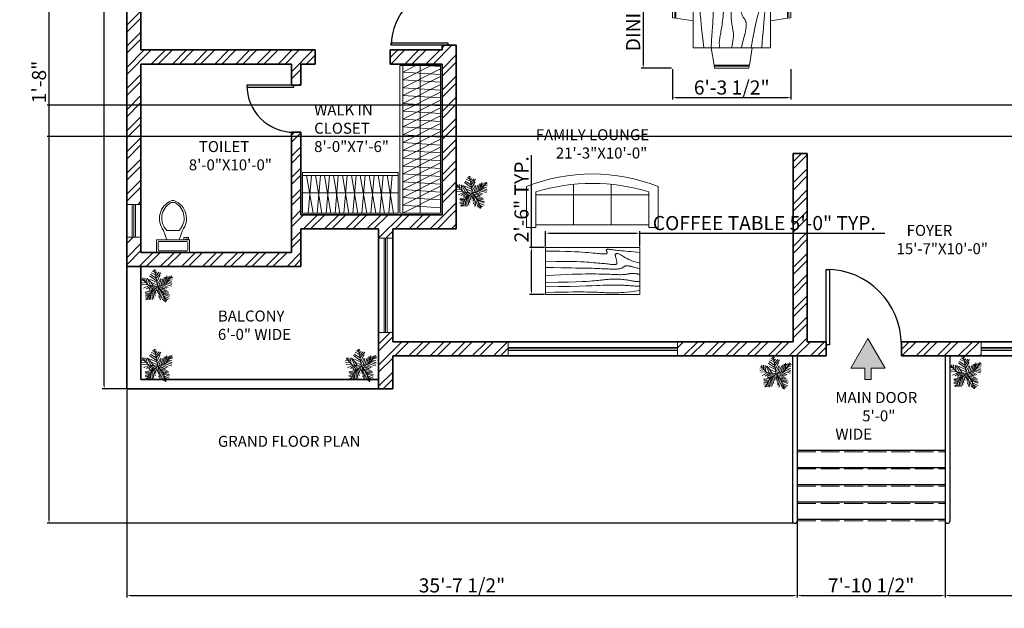
# Model space of a CAD drawing. Units: inches. Extents: x 416 to 1422, y 799 to 1634.
# Tile 1 of 5: x 416 to 1043, y 799 to 1174. Entities that reach past the tile are written whole.
import ezdxf

# ---------------------------------------------------------------- set-up
doc = ezdxf.new("R2010")
doc.units = ezdxf.units.IN
doc.linetypes.add('ACAD_ISO02W100', pattern=[15, 12, -3])
for name, color, linetype, lineweight in [('A-ANNO-DIMS', 2, 'Continuous', 18), ('A-ANNO-SYMB', 7, 'Continuous', 18), ('A-ANNO-TEXT', 7, 'Continuous', 18), ('A-AREA-IDEN', 7, 'Continuous', 18), ('A-DOOR', 4, 'Continuous', 25), ('A-FLOR-CASE', 8, 'Continuous', 18), ('A-FLOR-CASE-PATT', 252, 'Continuous', 13), ('A-FLOR-FIXT', 9, 'Continuous', 18), ('A-FLOR-STRS', 7, 'Continuous', 25), ('A-FLOR-STRS-HIDN', 8, 'ACAD_ISO02W100', 13), ('A-FURN', 8, 'Continuous', 18), ('A-GLAZ', 244, 'Continuous', 18), ('A-WALL', 7, 'Continuous', 35), ('A-WALL-PATT', 252, 'Continuous', 13), ('L-PLNT', 3, 'Continuous', 13)]:
    doc.layers.add(name, color=color, linetype=linetype, lineweight=lineweight)
doc.styles.get("Standard").update_dxf_attribs({"font": 'arial.ttf'})
doc.dimstyles.new('ISO-25', dxfattribs={"dimtxt": 9, "dimasz": 2.5, "dimexe": 1.25, "dimexo": 0.625, "dimtad": 1, "dimlunit": 3, "dimtxsty": 'Standard', "dimcen": 2.5, "dimadec": 0, "dimazin": 0, "dimtfac": 1, "dimtmove": 0, "dimatfit": 3, "dimfxl": 1, "dimarcsym": 0})

# ---------------------------------------------------------------- blocks, each defined once
blk = doc.blocks.new('*U2')
for p, q in [((0, 0), (0, -6)), ((40, 0), (40, -6))]:
    blk.add_line(p, q)
blk.add_lwpolyline([(0, 0), (0, 40), (1.75, 40), (1.75, 0)], close=True)
blk.add_arc((0, 0), 40, 0, 90)
blk = doc.blocks.new('*U8')
for p, q in [((0, 0), (0, -6)), ((-40, 0), (-40, -6))]:
    blk.add_line(p, q)
blk.add_lwpolyline([(0, 0), (0, 40), (-1.75, 40), (-1.75, 0)], close=True)
blk.add_arc((0, 0), 40, 90, 180)
blk = doc.blocks.new('*U7')
for p, q in [((9.5, -6), (9.5, -2)), ((-10, -8.5), (-8, -8.5)), ((-10, -9.5), (-10, -8.5)), ((-7, -9.5), (-10, -9.5)), ((-8, -8.5), (-8, -8)), ((-7, -8), (-7, -9.5)), ((-4, -8), (-6, -14)), ((4, -8), (6, -14)), ((4, -14), (-4, -14))]:
    blk.add_line(p, q)
blk.add_lwpolyline([(10.5, -8), (10.5, 0), (-10.5, 0), (-10.5, -8)], close=True)
for points in [[(-9.5, -2), (-9.5, -6)], [(8.5, -1), (-8.5, -1)], [(-8.5, -7), (8.5, -7)]]:
    blk.add_lwpolyline(points)
for centre, radius, start, end in [((-8.62, -1.88), 0.884, 81.8699, 188.1301), ((-8.62, -6.12), 0.884, 171.8699, 278.1301), ((8.62, -1.88), 0.884, 351.8699, 98.1301), ((8.62, -6.12), 0.884, 261.8699, 8.1301), ((3.52, -21.58), 12.17, 141.46911, 247.97143), ((4.2, -21.82), 11.33, 136.36773, 238.94682), ((-3.52, -21.58), 12.17, 292.02843, 38.53071), ((-4.2, -21.82), 11.33, 301.05301, 43.63209), ((0, -27.88), 4, 245.73182, 294.26817), ((0, -29), 4, 254.86053, 285.13947)]:
    blk.add_arc(centre, radius, start, end)
blk = doc.blocks.new('Dining Set - 36 x 72 in.')
for p, q in [((-22, 27.5), (-22.1562, 26.50042)), ((-22, 27.5), (-6, 27.5)), ((-5.8437, 26.49966), (-6, 27.5)), ((6, 27.5), (5.8438, 26.50042)), ((6, 27.5), (22, 27.5)), ((22.1563, 26.49966), (22, 27.5)), ((-22.2343, 26.00059), (-23.4847, 17.99762)), ((-22.2304, 26), (-5.7608, 26)), ((-5.8416, 26.5), (-22.1534, 26.5)), ((-4.5152, 17.99762), (-5.7655, 25.99926)), ((5.7657, 26.00059), (4.5153, 17.99762)), ((5.7696, 26), (22.2392, 26)), ((22.1584, 26.5), (5.8466, 26.5)), ((23.4848, 17.99762), (22.2345, 25.99926)), ((36, 18), (-36, 18)), ((-36, 18), (-36, -18)), ((36, -18), (36, 18)), ((-44.0006, 8.23428), (-35.9976, 9.48474)), ((44.0006, 8.23428), (35.9976, 9.48474)), ((-45.5, 8), (-44.5004, 8.15617)), ((-45.5, 8), (-45.5, -8)), ((-44.5, -8.15843), (-44.5, 8.15338)), ((-44, 8.23041), (-44, -8.23915)), ((44, 8.23041), (44, -8.23915)), ((44.5, -8.15843), (44.5, 8.15338)), ((45.5, 8), (44.5005, 8.15617)), ((45.5, 8), (45.5, -8)), ((-44.4997, -8.15631), (-45.5, -8)), ((-35.9976, -9.48476), (-43.9993, -8.2345)), ((35.9976, -9.48476), (43.9993, -8.2345)), ((44.4997, -8.15631), (45.5, -8)), ((-36, -18), (36, -18)), ((-22.2343, -26.0006), (-23.4847, -17.99762)), ((-4.5152, -17.99762), (-5.7655, -25.99928)), ((5.7657, -26.0006), (4.5153, -17.99762)), ((23.4848, -17.99762), (22.2345, -25.99928)), ((-22.2304, -26), (-5.7608, -26)), ((-22, -27.5), (-22.1562, -26.50044)), ((-5.8416, -26.5), (-22.1534, -26.5)), ((-5.8437, -26.49967), (-6, -27.5)), ((5.7696, -26), (22.2392, -26)), ((6, -27.5), (5.8438, -26.50044)), ((22.1584, -26.5), (5.8466, -26.5)), ((22.1563, -26.49967), (22, -27.5)), ((-22, -27.5), (-6, -27.5)), ((6, -27.5), (22, -27.5))]:
    blk.add_line(p, q)
for points in [[(-36, 15), (-31.1772, 14.97754), (-26.8079, 14.91406), (-22.8538, 14.81543), (-19.276, 14.6875), (-16.0362, 14.53613), (-13.0957, 14.36718), (-10.4159, 14.18652), (-7.9583, 14), (-5.6904, 13.81315), (-3.6035, 13.63021), (-1.6954, 13.45508), (0.0365, 13.29166), (1.5945, 13.14388), (2.9811, 13.01562), (4.1988, 12.9108), (5.25, 12.83333), (6.1393, 12.78613), (6.8802, 12.76823), (7.4883, 12.77767), (7.9792, 12.8125), (8.3685, 12.87077), (8.6719, 12.95052), (8.9049, 13.0498), (9.0833, 13.16666), (9.2205, 13.29899), (9.3216, 13.44401), (9.3895, 13.59879), (9.4271, 13.76041), (9.4373, 13.92594), (9.4232, 14.09245), (9.3875, 14.257), (9.3333, 14.41666), (9.2638, 14.56917), (9.1836, 14.71484), (9.0975, 14.85465), (9.0104, 14.98958), (8.9272, 15.1206), (8.8529, 15.2487), (8.7922, 15.37483), (8.75, 15.5), (8.7305, 15.62467), (8.7344, 15.74739), (8.7617, 15.86621), (8.8125, 15.97916), (8.8867, 16.08431), (8.9844, 16.17968), (9.1055, 16.26334), (9.25, 16.33333), (9.4189, 16.38802), (9.6172, 16.42708), (9.8506, 16.45052), (10.125, 16.45833), (10.4463, 16.45052), (10.8203, 16.42708), (11.2529, 16.38802), (11.75, 16.33333), (12.3184, 16.26318), (12.9694, 16.17838), (13.7151, 16.07991), (14.5677, 15.96875), (15.5395, 15.84586), (16.6426, 15.71224), (17.8893, 15.56884), (19.2917, 15.41666), (20.859, 15.25667), (22.5879, 15.08984), (24.4721, 14.91715), (26.5052, 14.73958), (28.6809, 14.5581), (30.9929, 14.3737), (33.4347, 14.18733), (36, 14)], [(-36, 10), (-28.9766, 10.14274), (-23.1725, 10.20442), (-18.4241, 10.19775), (-14.5677, 10.13541), (-11.4399, 10.03011), (-8.877, 9.89453), (-6.7154, 9.74137), (-4.7917, 9.58333), (-2.9698, 9.43082), (-1.2246, 9.28515), (0.4415, 9.14534), (2.026, 9.01041), (3.5266, 8.87939), (4.9408, 8.7513), (6.266, 8.62516), (7.5, 8.5), (8.6411, 8.37549), (9.6914, 8.2539), (10.6538, 8.13818), (11.5312, 8.03125), (12.3267, 7.93603), (13.043, 7.85547), (13.6831, 7.79248), (14.25, 7.75), (14.7471, 7.7303), (15.1797, 7.73307), (15.5537, 7.75732), (15.875, 7.80208), (16.1494, 7.86637), (16.3828, 7.94922), (16.5811, 8.04964), (16.75, 8.16666), (16.8944, 8.29915), (17.0143, 8.44531), (17.1089, 8.60319), (17.1771, 8.77083), (17.218, 8.94629), (17.2305, 9.1276), (17.2137, 9.31282), (17.1667, 9.5), (17.0895, 9.6875), (16.987, 9.875), (16.8649, 10.0625), (16.7292, 10.25), (16.5856, 10.4375), (16.4401, 10.625), (16.2985, 10.8125), (16.1667, 11), (16.05, 11.18733), (15.9518, 11.3737), (15.8752, 11.5581), (15.8229, 11.73958), (15.798, 11.91715), (15.8034, 12.08984), (15.842, 12.25667), (15.9167, 12.41666), (16.0295, 12.56836), (16.1784, 12.70833), (16.3605, 12.83268), (16.5729, 12.9375), (16.8127, 13.01888), (17.0768, 13.07291), (17.3625, 13.0957), (17.6667, 13.08333), (17.9894, 13.03312), (18.3418, 12.94726), (18.7382, 12.82918), (19.1927, 12.68229), (19.7195, 12.51001), (20.3327, 12.31575), (21.0465, 12.10294), (21.875, 11.875), (22.8357, 11.63354), (23.959, 11.37304), (25.2786, 11.08618), (26.8282, 10.76562), (28.6414, 10.40405), (30.752, 9.99414), (33.1936, 9.52856), (36, 9)], [(-36, 5.5), (-30.7157, 5.3348), (-26.069, 5.20963), (-21.9946, 5.11767), (-18.4271, 5.05208), (-15.3009, 5.00602), (-12.5508, 4.97265), (-10.1112, 4.94515), (-7.9167, 4.91666), (-5.909, 4.88167), (-4.0586, 4.83984), (-2.3429, 4.79215), (-0.7396, 4.73958), (0.7739, 4.6831), (2.22, 4.6237), (3.6213, 4.56233), (5, 4.5), (6.373, 4.43782), (7.7344, 4.3776), (9.0723, 4.32129), (10.375, 4.27083), (11.6309, 4.22819), (12.8281, 4.19531), (13.9551, 4.17415), (15, 4.16666), (15.954, 4.17448), (16.819, 4.19791), (17.6001, 4.23698), (18.3021, 4.29166), (18.9299, 4.36198), (19.4883, 4.44791), (19.9823, 4.54948), (20.4167, 4.66666), (20.7969, 4.79899), (21.1302, 4.94401), (21.4245, 5.09879), (21.6875, 5.26041), (21.9271, 5.42594), (22.1511, 5.59245), (22.3672, 5.757), (22.5834, 5.91666), (22.8065, 6.06868), (23.0404, 6.21093), (23.2879, 6.34147), (23.5521, 6.45833), (23.8358, 6.55957), (24.142, 6.64323), (24.4735, 6.70735), (24.8334, 6.75), (25.2235, 6.76969), (25.642, 6.76692), (26.0858, 6.74267), (26.5521, 6.69791), (27.0379, 6.63362), (27.5404, 6.55078), (28.0565, 6.45036), (28.5834, 6.33333), (29.1242, 6.19987), (29.7071, 6.04687), (30.3661, 5.87044), (31.1354, 5.66666), (32.0493, 5.43164), (33.142, 5.16146), (34.4475, 4.85221), (36, 4.5)], [(-36, -1), (-30.7915, -0.6591), (-26.0195, -0.38216), (-21.6519, -0.16284), (-17.6563, 0.00521), (-14.0005, 0.12833), (-10.6523, 0.21289), (-7.5796, 0.26522), (-4.75, 0.29166), (-2.134, 0.29793), (0.2878, 0.28711), (2.5317, 0.26163), (4.6146, 0.22396), (6.5529, 0.17651), (8.3633, 0.12174), (10.0623, 0.06209), (11.6667, 0), (13.1899, -0.06201), (14.6341, -0.1211), (15.9982, -0.17432), (17.2813, -0.21875), (18.4823, -0.25147), (19.6003, -0.26953), (20.6343, -0.27002), (21.5834, -0.25), (22.4481, -0.20768), (23.2357, -0.14584), (23.9549, -0.06836), (24.6146, 0.02083), (25.2235, 0.11784), (25.7904, 0.21875), (26.3241, 0.31966), (26.8334, 0.41666), (27.3265, 0.50618), (27.8099, 0.58593), (28.2894, 0.65397), (28.7709, 0.70833), (29.2601, 0.74707), (29.763, 0.76823), (30.2855, 0.76985), (30.8334, 0.75), (31.4088, 0.70784), (31.9994, 0.64713), (32.589, 0.57275), (33.1615, 0.48958), (33.7008, 0.4025), (34.1908, 0.3164), (34.6153, 0.23616), (34.9584, 0.16666), (35.2099, 0.11165), (35.3848, 0.07031), (35.504, 0.04069), (35.5886, 0.02083), (35.6594, 0.00879), (35.7377, 0.0026), (35.8442, 0.00032), (36, 0)], [(-36, -6.5), (-27.1843, -6.31267), (-20.084, -6.1263), (-14.469, -5.9419), (-10.1094, -5.76042), (-6.7752, -5.58285), (-4.2363, -5.41016), (-2.2629, -5.24333), (-0.625, -5.08334), (0.8708, -4.93099), (2.2715, -4.78646), (3.5872, -4.64974), (4.8281, -4.52084), (6.0046, -4.39974), (7.127, -4.28646), (8.2053, -4.18099), (9.25, -4.08334), (10.2705, -3.99382), (11.2734, -3.91407), (12.2647, -3.84603), (13.25, -3.79167), (14.2354, -3.75293), (15.2266, -3.73177), (16.2295, -3.73015), (17.25, -3.75), (18.2912, -3.79248), (19.3451, -3.85547), (20.4009, -3.93604), (21.4479, -4.03125), (22.4754, -4.13819), (23.4727, -4.25391), (24.4289, -4.37549), (25.3334, -4.5), (26.1785, -4.62492), (26.9694, -4.74935), (27.7145, -4.87281), (28.4219, -4.99479), (29.1, -5.11483), (29.7572, -5.23242), (30.4016, -5.34709), (31.0417, -5.45834), (31.6837, -5.56437), (32.3262, -5.65821), (32.9658, -5.73153), (33.599, -5.77604), (34.2224, -5.78345), (34.8327, -5.74545), (35.4264, -5.65373), (36, -5.5)], [(-36, -10), (-26.4022, -9.81299), (-18.4675, -9.62891), (-11.9839, -9.45069), (-6.7396, -9.28125), (-2.5226, -9.12354), (0.8789, -8.98047), (3.6769, -8.85498), (6.0833, -8.75), (8.2767, -8.66765), (10.3021, -8.60677), (12.1712, -8.56543), (13.8958, -8.54167), (15.4876, -8.53353), (16.9583, -8.53907), (18.3197, -8.55632), (19.5834, -8.58334), (20.7616, -8.61841), (21.8685, -8.66081), (22.9188, -8.71004), (23.9271, -8.76563), (24.9081, -8.82707), (25.8763, -8.89388), (26.8465, -8.96558), (27.8334, -9.04167), (28.8474, -9.12118), (29.8828, -9.20117), (30.93, -9.27824), (31.9792, -9.34896), (33.0205, -9.40991), (34.0443, -9.45768), (35.0407, -9.48885), (36, -9.5)], [(-36, -14.5), (-30.0881, -14.33513), (-25.0332, -14.21224), (-20.7312, -14.12647), (-17.0781, -14.07292), (-13.97, -14.04671), (-11.3027, -14.04297), (-8.9724, -14.05681), (-6.875, -14.08334), (-4.9224, -14.11833), (-3.0905, -14.16016), (-1.3709, -14.20785), (0.2448, -14.26042), (1.7647, -14.3169), (3.1973, -14.3763), (4.5507, -14.43767), (5.8333, -14.5), (7.0554, -14.5621), (8.235, -14.62175), (9.3922, -14.67652), (10.5469, -14.72396), (11.7192, -14.76164), (12.929, -14.78711), (14.1965, -14.79794), (15.5417, -14.79167), (16.9933, -14.76424), (18.6152, -14.70508), (20.4804, -14.60197), (22.6615, -14.44271), (25.2312, -14.21509), (28.2624, -13.9069), (31.8277, -13.50594), (36, -13)]]:
    blk.add_lwpolyline(points)
blk = doc.blocks.new('Sofa - Roundback 7 ft.')
for p, q in [((-36.000027, -34), (-36.000027, -11.4696)), ((-12.00002, -32.4421), (-12.00003, -6.5971)), ((11.99997, -32.4421), (11.99998, -6.5971)), ((35.99998, -34), (35.99998, -11.4696)), ((-35.999844, -13.3819), (35.9998, -13.3819)), ((-36.000027, -32.4421), (35.99998, -32.4421))]:
    blk.add_line(p, q)
for points in [[(-36.000027, -34), (-42.000027, -34), (-42.000027, -8)], [(41.99998, -8), (41.99998, -34), (35.99998, -34)]]:
    blk.add_lwpolyline(points)
for centre, radius, start, end in [((0, -114.25), 114.25, 68.43141, 111.5686), ((-0.00001, -127.1968), 121.1968, 72.72033, 107.2797)]:
    blk.add_arc(centre, radius, start, end)
blk = doc.blocks.new('Table - Rectangular Woodgrain 60 x 30 in.')
for p, q in [((0, 0), (0, -30)), ((60, 0), (0, 0)), ((60, -30), (60, 0)), ((0, -30), (60, -30))]:
    blk.add_line(p, q)
for points in [[(0, -2.4), (4.8155, -2.418), (9.0302, -2.4688), (12.709, -2.5477), (15.9167, -2.65), (18.7181, -2.7711), (21.1781, -2.9063), (23.3616, -3.0508), (25.3333, -3.2), (27.1477, -3.3495), (28.8172, -3.4958), (30.3437, -3.636), (31.7291, -3.7667), (32.9756, -3.8849), (34.0849, -3.9875), (35.059, -4.0714), (35.9, -4.1334), (36.6114, -4.1711), (37.2041, -4.1854), (37.6906, -4.1779), (38.0833, -4.15), (38.3948, -4.1034), (38.6375, -4.0396), (38.8239, -3.9602), (38.9666, -3.8667), (39.0764, -3.7608), (39.1573, -3.6448), (39.2116, -3.521), (39.2416, -3.3917), (39.2498, -3.2593), (39.2385, -3.1261), (39.21, -2.9944), (39.1666, -2.8667), (39.111, -2.7447), (39.0468, -2.6281), (38.978, -2.5163), (38.9083, -2.4083), (38.8418, -2.3035), (38.7823, -2.201), (38.7337, -2.1001), (38.7, -2), (38.6844, -1.9003), (38.6875, -1.8021), (38.7094, -1.707), (38.75, -1.6167), (38.8094, -1.5326), (38.8875, -1.4563), (38.9844, -1.3893), (39.1, -1.3333), (39.2351, -1.2896), (39.3937, -1.2583), (39.5804, -1.2396), (39.8, -1.2333), (40.057, -1.2396), (40.3562, -1.2583), (40.7023, -1.2896), (41.1, -1.3333), (41.5547, -1.3895), (42.0755, -1.4573), (42.6721, -1.5361), (43.3542, -1.625), (44.1316, -1.7233), (45.014, -1.8302), (46.0114, -1.9449), (47.1333, -2.0667), (48.3862, -2.1947), (49.7625, -2.3281), (51.2513, -2.4663), (52.8416, -2.6083), (54.5226, -2.7535), (56.2833, -2.9011), (58.1127, -3.0501), (60, -3.2)], [(0, -9.2), (6.5759, -9.0858), (11.9385, -9.0365), (16.2527, -9.0418), (19.6833, -9.0917), (22.3952, -9.1759), (24.5531, -9.2844), (26.322, -9.4069), (27.8666, -9.5333), (29.3241, -9.6553), (30.7203, -9.7719), (32.0532, -9.8837), (33.3208, -9.9917), (34.5213, -10.0965), (35.6526, -10.199), (36.7128, -10.2999), (37.7, -10.4), (38.6129, -10.4996), (39.4531, -10.5969), (40.223, -10.6895), (40.925, -10.775), (41.5613, -10.8512), (42.1344, -10.9156), (42.6465, -10.966), (43.1, -11), (43.4976, -11.0158), (43.8437, -11.0136), (44.143, -10.9942), (44.4, -10.9583), (44.6195, -10.9069), (44.8062, -10.8406), (44.9648, -10.7603), (45.1, -10.6667), (45.2155, -10.5598), (45.3114, -10.4365), (45.3871, -10.2929), (45.4416, -10.125), (45.4743, -9.929), (45.4844, -9.7011), (45.4709, -9.4371), (45.4333, -9.1333), (45.3716, -8.7883), (45.2896, -8.4104), (45.1919, -8.0107), (45.0833, -7.6), (44.9685, -7.1893), (44.8521, -6.7896), (44.7388, -6.4117), (44.6333, -6.0667), (44.54, -5.7628), (44.4614, -5.4979), (44.4001, -5.2675), (44.3583, -5.0667), (44.3384, -4.8909), (44.3427, -4.7354), (44.3736, -4.5956), (44.4333, -4.4667), (44.5236, -4.3453), (44.6427, -4.2333), (44.7884, -4.1339), (44.9583, -4.05), (45.1501, -3.9849), (45.3614, -3.9417), (45.59, -3.9234), (45.8333, -3.9333), (46.0915, -3.9749), (46.3734, -4.0531), (46.6906, -4.1736), (47.0542, -4.3417), (47.4756, -4.5629), (47.9661, -4.8427), (48.5372, -5.1866), (49.2, -5.6), (49.9676, -6.0844), (50.8594, -6.625), (51.8965, -7.2031), (53.1, -7.8), (54.491, -8.3969), (56.0906, -8.975), (57.9199, -9.5156), (60, -10)], [(0, -12.8), (5.1847, -12.9322), (9.6213, -13.0323), (13.3963, -13.1059), (16.5958, -13.1583), (19.3063, -13.1952), (21.614, -13.2219), (23.6054, -13.2439), (25.3666, -13.2667), (26.9728, -13.2947), (28.4531, -13.3281), (29.8256, -13.3663), (31.1083, -13.4083), (32.3191, -13.4535), (33.476, -13.501), (34.597, -13.5501), (35.7, -13.6), (36.7984, -13.6497), (37.8875, -13.6979), (38.9578, -13.743), (40, -13.7833), (41.0047, -13.8174), (41.9625, -13.8438), (42.864, -13.8607), (43.7, -13.8667), (44.4631, -13.8604), (45.1552, -13.8417), (45.7801, -13.8104), (46.3416, -13.7667), (46.8439, -13.7104), (47.2906, -13.6417), (47.6858, -13.5604), (48.0333, -13.4667), (48.3375, -13.3608), (48.6042, -13.2448), (48.8396, -13.121), (49.05, -12.9917), (49.2417, -12.8593), (49.4208, -12.7261), (49.5937, -12.5944), (49.7667, -12.4667), (49.9452, -12.3451), (50.1323, -12.2313), (50.3303, -12.1268), (50.5416, -12.0333), (50.7686, -11.9524), (51.0135, -11.8854), (51.2788, -11.8341), (51.5666, -11.8), (51.8785, -11.7843), (52.2116, -11.7865), (52.562, -11.8059), (52.926, -11.8417), (53.2998, -11.8931), (53.6795, -11.9594), (54.0614, -12.0397), (54.4416, -12.1333), (54.8223, -12.2401), (55.2293, -12.3625), (55.6942, -12.5037), (56.2489, -12.6667), (56.9251, -12.8547), (57.7545, -13.0708), (58.7689, -13.3182), (60, -13.6)], [(0, -18), (5.124, -17.7273), (9.6609, -17.5057), (13.6705, -17.3303), (17.2125, -17.1958), (20.3467, -17.0973), (23.1328, -17.0297), (25.6307, -16.9878), (27.9, -16.9667), (29.9928, -16.9617), (31.9302, -16.9703), (33.7254, -16.9907), (35.3917, -17.0208), (36.9423, -17.0588), (38.3906, -17.1026), (39.7499, -17.1503), (41.0333, -17.2), (42.2519, -17.2496), (43.4073, -17.2969), (44.4986, -17.3395), (45.525, -17.375), (46.4858, -17.4012), (47.3802, -17.4156), (48.2074, -17.416), (48.9667, -17.4), (49.6583, -17.3662), (50.2872, -17.3167), (50.8595, -17.2547), (51.3812, -17.1833), (51.8584, -17.1057), (52.2971, -17.025), (52.7034, -16.9443), (53.0833, -16.8667), (53.443, -16.7951), (53.789, -16.7313), (54.128, -16.6768), (54.4666, -16.6334), (54.8115, -16.6024), (55.1693, -16.5854), (55.5465, -16.5841), (55.95, -16.6), (56.3828, -16.6337), (56.8346, -16.6823), (57.2915, -16.7418), (57.7396, -16.8084), (58.165, -16.878), (58.5539, -16.9469), (58.8924, -17.0111), (59.1666, -17.0667), (59.3679, -17.1107), (59.5078, -17.1438), (59.6032, -17.1675), (59.6708, -17.1833), (59.7275, -17.193), (59.7901, -17.1979), (59.8753, -17.1998), (60, -17.2)], [(0, -22.4), (8.0098, -22.2501), (14.4094, -22.1011), (19.4168, -21.9535), (23.25, -21.8083), (26.1269, -21.6663), (28.2656, -21.5281), (29.884, -21.3947), (31.2, -21.2667), (32.3967, -21.1448), (33.5172, -21.0292), (34.5697, -20.9198), (35.5625, -20.8167), (36.5037, -20.7198), (37.4015, -20.6292), (38.2642, -20.5448), (39.1, -20.4667), (39.9164, -20.3951), (40.7187, -20.3313), (41.5117, -20.2768), (42.3, -20.2333), (43.0883, -20.2024), (43.8812, -20.1854), (44.6836, -20.1841), (45.5, -20.2), (46.3328, -20.234), (47.1747, -20.2844), (48.0163, -20.3488), (48.8479, -20.425), (49.66, -20.5106), (50.4429, -20.6031), (51.1872, -20.7004), (51.8833, -20.8), (52.5246, -20.8999), (53.1166, -20.9995), (53.6681, -21.0983), (54.1875, -21.1958), (54.6834, -21.2919), (55.1646, -21.3859), (55.6394, -21.4777), (56.1167, -21.5667), (56.6028, -21.6515), (57.0961, -21.7266), (57.5929, -21.7852), (58.0896, -21.8208), (58.5823, -21.8268), (59.0674, -21.7964), (59.5412, -21.723), (60, -21.6)], [(0, -25.2), (8.6355, -25.0504), (15.7026, -24.9031), (21.4049, -24.7606), (25.9458, -24.625), (29.529, -24.4988), (32.3578, -24.3844), (34.6359, -24.284), (36.5667, -24.2), (38.3213, -24.1341), (39.9417, -24.0854), (41.437, -24.0523), (42.8167, -24.0333), (44.0901, -24.0268), (45.2667, -24.0313), (46.3557, -24.0451), (47.3667, -24.0667), (48.309, -24.0947), (49.1928, -24.1287), (50.0284, -24.168), (50.826, -24.2125), (51.5959, -24.2617), (52.3483, -24.3151), (53.0935, -24.3725), (53.8417, -24.4334), (54.6009, -24.497), (55.3699, -24.561), (56.1454, -24.6226), (56.9239, -24.6792), (57.7021, -24.7279), (58.4764, -24.7662), (59.2435, -24.7911), (60, -24.8)], [(0, -28.8), (5.6867, -28.6681), (10.45, -28.5698), (14.407, -28.5012), (17.675, -28.4584), (20.3711, -28.4374), (22.6125, -28.4344), (24.5164, -28.4455), (26.2, -28.4667), (27.762, -28.4947), (29.2276, -28.5281), (30.6033, -28.5663), (31.8958, -28.6084), (33.1118, -28.6535), (34.2578, -28.7011), (35.3405, -28.7501), (36.3666, -28.8), (37.3443, -28.8497), (38.288, -28.8974), (39.2137, -28.9412), (40.1375, -28.9792), (41.0753, -29.0093), (42.0432, -29.0297), (43.0572, -29.0384), (44.1333, -29.0333), (45.2936, -29.0114), (46.5843, -28.9641), (48.0579, -28.8816), (49.7666, -28.7542), (51.7629, -28.5721), (54.0989, -28.3255), (56.8272, -28.0048), (60, -27.6)]]:
    blk.add_lwpolyline(points)
blk = doc.blocks.new('*U15')
for p, q in [((-3.665, 19.273), (-27.574, 35.527)), ((-5.114, 28.097), (-24.676, 40.636)), ((-7.288, 39.707), (-21.778, 46.673)), ((-8.737, 47.138), (-17.069, 52.711)), ((-10.186, 53.64), (-13.084, 55.962)), ((0, 0), (-10.5, 57)), ((-9.099, 51.782), (-6.563, 55.962)), ((-7.65, 43.423), (-2.578, 49.46)), ((-5.839, 35.992), (4.667, 48.067)), ((-5.114, 27.632), (10.463, 46.673)), ((-2.941, 16.486), (8.652, 37.85)), ((27, 9), (48, 36)), ((27.127, 9.056), (31.112, 35.992)), ((38.719, 34.134), (41.979, 28.561)), ((44.153, 36.456), (45.239, 32.741)), ((-47.498, 19.737), (-55.83, 18.344)), ((-40.615, 13.7), (-55.105, 10.913)), ((-31.5, 4.5), (-52.5, 25.5)), ((-33.37, 6.269), (-52.207, 5.34)), ((-48.585, 21.131), (-49.309, 29.026)), ((-28.299, 3.483), (-47.86, -5.805)), ((-43.513, 28.561), (-42.427, 15.558)), ((-38.442, 26.239), (-34.819, 7.663)), ((-21.416, 3.018), (-38.079, -8.128)), ((-35.544, 28.097), (-24.314, 3.947)), ((0, 0), (-31.5, 4.5)), ((-14.533, 2.09), (-30.834, 25.31)), ((-15.982, 2.09), (-30.11, -9.521)), ((-24.314, 23.917), (-2.941, 13.7)), ((0, 0), (-22.5, -19.5)), ((-6.563, 1.161), (-21.416, -8.128)), ((-20.691, 13.7), (-1.129, 4.876)), ((-1.129, 6.734), (9.014, 26.704)), ((0, 0), (27, 9)), ((0, 0), (18, -22.5)), ((3.942, 1.625), (11.187, 24.381)), ((6.478, 1.625), (26.04, -8.592)), ((10.101, 3.483), (17.708, 26.239)), ((11.187, 3.483), (30.749, -5.805)), ((16.259, 5.805), (23.142, 31.348)), ((18.07, 5.805), (35.096, -3.483)), ((22.055, 7.198), (27.489, 32.277)), ((24.229, 7.663), (46.688, 1.625)), ((29.662, 12.307), (48.137, 6.269)), ((31.836, 30.883), (32.561, 16.486)), ((33.285, 16.486), (48.862, 10.913)), ((35.096, 32.741), (37.27, 22.524)), ((36.183, 19.737), (48.137, 17.88)), ((40.53, 25.775), (48.862, 24.846)), ((43.791, 29.954), (51.036, 30.883)), ((-17.431, -15.094), (-42.789, -18.809)), ((-28.299, -29.026), (-42.789, -31.348)), ((-24.314, -21.596), (-42.427, -22.06)), ((-26.849, -26.24), (-40.253, -25.775)), ((-22.5, -19.5), (-37.5, -45)), ((-15.257, -12.772), (-30.11, -12.772)), ((-29.023, -30.884), (-27.936, -43.887)), ((-25.038, -23.918), (-22.865, -45.281)), ((-20.691, -18.345), (-17.793, -44.352)), ((-6.563, -5.805), (-19.967, -9.985)), ((-17.069, -15.094), (-12.721, -40.172)), ((-13.446, -11.378), (-8.737, -32.741)), ((-9.461, -8.592), (-6.201, -23.453)), ((-4.752, -3.483), (-3.665, -14.629)), ((2.493, -3.019), (-1.491, -20.202)), ((1.769, -2.555), (24.229, -9.521)), ((5.029, -6.27), (2.131, -25.775)), ((9.014, -11.378), (3.58, -35.992)), ((14.085, -16.951), (6.478, -40.172)), ((7.565, -9.056), (32.198, -14.629)), ((18.07, -22.524), (8.289, -45.745)), ((12.274, -15.094), (36.907, -18.809)), ((20.244, -30.419), (15.897, -44.816)), ((16.259, -19.738), (36.183, -22.989)), ((18, -22.5), (27, -52.5)), ((18.433, -22.524), (40.53, -29.026)), ((19.157, -25.311), (38.719, -33.206)), ((21.331, -32.741), (39.081, -40.636)), ((-30.834, -34.135), (-42.427, -35.528)), ((-34.457, -39.708), (-40.978, -42.494)), ((-32.646, -36.921), (-31.921, -44.352)), ((22.78, -37.85), (19.519, -48.532)), ((22.78, -38.314), (34.372, -44.816)), ((24.591, -45.745), (23.142, -50.854)), ((24.591, -43.423), (30.749, -47.603)), ((26.764, -49.925), (28.213, -50.854))]:
    blk.add_line(p, q)
blk = doc.blocks.new('*D16')
at = {"layer": 'A-ANNO-DIMS', "color": 0, "lineweight": -2, "transparency": 16777216}
for p, q in [((483.19, 1569.01), (468.17, 1569.01)), ((469.42, 941.51), (469.42, 1566.51)), ((483.19, 939.01), (468.17, 939.01))]:
    blk.add_line(p, q, dxfattribs=at)
at = {"layer": 'A-ANNO-DIMS', "color": 0, "transparency": 16777216}
for points in [[(469, 1566.51), (469.84, 1566.51), (469.42, 1569.01)], [(469, 941.51), (469.84, 941.51), (469.42, 939.01)]]:
    blk.add_solid(points, dxfattribs=at)
at = {"layer": 'Defpoints', "color": 0, "transparency": 16777216}
for p in [(469.42, 1569.01), (483.82, 1569.01), (483.82, 939.01)]:
    blk.add_point(p, dxfattribs=at)
at = {"layer": 'A-ANNO-DIMS', "color": 0, "transparency": 16777216, "insert": (464.2, 1254.01), "char_height": 9, "attachment_point": 5, "rotation": 90}
blk.add_mtext('52\'-6"', dxfattribs=at)
blk = doc.blocks.new('WIN-21IN')
for p, q in [((21, 5.5), (0, 5.5)), ((21, 4.5), (0, 4.5)), ((21, 3.5), (0, 3.5))]:
    blk.add_line(p, q)
blk.add_lwpolyline([(21, 9), (21, 0), (0, 0), (0, 9)], close=True)
blk = doc.blocks.new('WIN-60IN')
for p, q in [((3.5, 60), (3.5, 0)), ((4.5, 60), (4.5, 0)), ((5.5, 60), (5.5, 0))]:
    blk.add_line(p, q)
blk.add_lwpolyline([(0, 60), (9, 60), (9, 0), (0, 0)], close=True)
blk = doc.blocks.new('*D33')
at = {"layer": 'A-ANNO-DIMS', "color": 0, "lineweight": -2, "transparency": 16777216}
for p, q in [((750.81, 1029.86), (750.81, 1039.48)), ((753.31, 1038.23), (808.31, 1038.23)), ((810.81, 1029.86), (810.81, 1039.48)), ((810.81, 1038.23), (967.12, 1038.23))]:
    blk.add_line(p, q, dxfattribs=at)
at = {"layer": 'A-ANNO-DIMS', "color": 0, "transparency": 16777216}
for points in [[(753.31, 1038.65), (753.31, 1037.82), (750.81, 1038.23)], [(808.31, 1038.65), (808.31, 1037.82), (810.81, 1038.23)]]:
    blk.add_solid(points, dxfattribs=at)
at = {"layer": 'Defpoints', "color": 0, "transparency": 16777216}
for p in [(810.81, 1038.23), (750.81, 1029.23), (810.81, 1029.23)]:
    blk.add_point(p, dxfattribs=at)
at = {"layer": 'A-ANNO-DIMS', "color": 0, "transparency": 16777216, "insert": (890.21, 1043.51), "char_height": 9, "attachment_point": 5}
blk.add_mtext('COFFEE TABLE 5\'-0" TYP.', dxfattribs=at)
blk = doc.blocks.new('*D34')
at = {"layer": 'A-ANNO-DIMS', "color": 0, "lineweight": -2, "transparency": 16777216}
for p, q in [((741.81, 1029.23), (741.81, 1088)), ((750.18, 1029.23), (740.56, 1029.23)), ((741.81, 1001.73), (741.81, 1026.73)), ((750.18, 999.23), (740.56, 999.23))]:
    blk.add_line(p, q, dxfattribs=at)
at = {"layer": 'A-ANNO-DIMS', "color": 0, "transparency": 16777216}
for points in [[(741.39, 1026.73), (742.22, 1026.73), (741.81, 1029.23)], [(741.39, 1001.73), (742.22, 1001.73), (741.81, 999.23)]]:
    blk.add_solid(points, dxfattribs=at)
at = {"layer": 'Defpoints', "color": 0, "transparency": 16777216}
for p in [(741.81, 1029.23), (750.81, 1029.23), (750.81, 999.23)]:
    blk.add_point(p, dxfattribs=at)
at = {"layer": 'A-ANNO-DIMS', "color": 0, "transparency": 16777216, "insert": (736.59, 1059.86), "char_height": 9, "attachment_point": 5, "rotation": 90}
blk.add_mtext('2\'-6" TYP.', dxfattribs=at)
blk = doc.blocks.new('*D41')
at = {"layer": 'A-ANNO-DIMS', "color": 0, "lineweight": -2, "transparency": 16777216}
for p, q in [((831.14, 1268.11), (811.8, 1268.11)), ((813.05, 1265.61), (813.05, 1145.85)), ((831.14, 1143.35), (811.8, 1143.35))]:
    blk.add_line(p, q, dxfattribs=at)
at = {"layer": 'A-ANNO-DIMS', "color": 0, "transparency": 16777216}
for points in [[(812.63, 1265.61), (813.46, 1265.61), (813.05, 1268.11)], [(812.63, 1145.85), (813.46, 1145.85), (813.05, 1143.35)]]:
    blk.add_solid(points, dxfattribs=at)
at = {"layer": 'Defpoints', "color": 0, "transparency": 16777216}
for p in [(831.76, 1268.11), (813.05, 1143.35), (831.76, 1143.35)]:
    blk.add_point(p, dxfattribs=at)
at = {"layer": 'A-ANNO-DIMS', "color": 0, "transparency": 16777216, "insert": (807.77, 1205.73), "char_height": 9, "attachment_point": 5, "rotation": 90}
blk.add_mtext('DINING SET 10\'-5"', dxfattribs=at)
blk = doc.blocks.new('*D42')
at = {"layer": 'A-ANNO-DIMS', "color": 0, "lineweight": -2, "transparency": 16777216}
for p, q in [((831.76, 1142.72), (831.76, 1123.38)), ((907.17, 1142.72), (907.17, 1123.38)), ((834.26, 1124.63), (904.67, 1124.63))]:
    blk.add_line(p, q, dxfattribs=at)
at = {"layer": 'A-ANNO-DIMS', "color": 0, "transparency": 16777216}
for points in [[(834.26, 1125.05), (834.26, 1124.21), (831.76, 1124.63)], [(904.67, 1125.05), (904.67, 1124.21), (907.17, 1124.63)]]:
    blk.add_solid(points, dxfattribs=at)
at = {"layer": 'Defpoints', "color": 0, "transparency": 16777216}
for p in [(831.76, 1143.35), (907.17, 1143.35), (907.17, 1124.63)]:
    blk.add_point(p, dxfattribs=at)
at = {"layer": 'A-ANNO-DIMS', "color": 0, "transparency": 16777216, "insert": (869.46, 1129.91), "char_height": 9, "attachment_point": 5}
blk.add_mtext('6\'-3 1/2"', dxfattribs=at)
blk = doc.blocks.new('*D43')
at = {"layer": 'A-ANNO-DIMS', "color": 0, "lineweight": -2, "transparency": 16777216}
for p, q in [((483.19, 1569.01), (433, 1569.01)), ((434.25, 855.88), (434.25, 1566.51)), ((909.15, 853.38), (433, 853.38))]:
    blk.add_line(p, q, dxfattribs=at)
at = {"layer": 'A-ANNO-DIMS', "color": 0, "transparency": 16777216}
for points in [[(433.83, 1566.51), (434.67, 1566.51), (434.25, 1569.01)], [(433.83, 855.88), (434.67, 855.88), (434.25, 853.38)]]:
    blk.add_solid(points, dxfattribs=at)
at = {"layer": 'Defpoints', "color": 0, "transparency": 16777216}
for p in [(434.25, 1569.01), (483.82, 1569.01), (909.77, 853.38)]:
    blk.add_point(p, dxfattribs=at)
at = {"layer": 'A-ANNO-DIMS', "color": 0, "transparency": 16777216, "insert": (428.97, 1211.2), "char_height": 9, "attachment_point": 5, "rotation": 90}
blk.add_mtext('59\'-7 1/2"', dxfattribs=at)
blk = doc.blocks.new('*D44')
at = {"layer": 'A-ANNO-DIMS', "color": 0, "lineweight": -2, "transparency": 16777216}
for p, q in [((483.82, 938.39), (483.82, 806.13)), ((911.18, 855.39), (911.18, 806.13)), ((486.32, 807.38), (908.68, 807.38))]:
    blk.add_line(p, q, dxfattribs=at)
at = {"layer": 'A-ANNO-DIMS', "color": 0, "transparency": 16777216}
for points in [[(486.32, 807.79), (486.32, 806.96), (483.82, 807.38)], [(908.68, 807.79), (908.68, 806.96), (911.18, 807.38)]]:
    blk.add_solid(points, dxfattribs=at)
at = {"layer": 'Defpoints', "color": 0, "transparency": 16777216}
for p in [(483.82, 939.01), (911.18, 856.01), (911.18, 807.38)]:
    blk.add_point(p, dxfattribs=at)
at = {"layer": 'A-ANNO-DIMS', "color": 0, "transparency": 16777216, "insert": (697.5, 812.66), "char_height": 9, "attachment_point": 5}
blk.add_mtext('35\'-7 1/2"', dxfattribs=at)
blk = doc.blocks.new('*D45')
at = {"layer": 'A-ANNO-DIMS', "color": 0, "lineweight": -2, "transparency": 16777216}
for p, q in [((911.18, 855.39), (911.18, 806.13)), ((1005.49, 855.39), (1005.49, 806.13)), ((913.68, 807.38), (1002.99, 807.38))]:
    blk.add_line(p, q, dxfattribs=at)
at = {"layer": 'A-ANNO-DIMS', "color": 0, "transparency": 16777216}
for points in [[(913.68, 807.79), (913.68, 806.96), (911.18, 807.38)], [(1002.99, 807.79), (1002.99, 806.96), (1005.49, 807.38)]]:
    blk.add_solid(points, dxfattribs=at)
at = {"layer": 'Defpoints', "color": 0, "transparency": 16777216}
for p in [(911.18, 856.01), (1005.49, 856.01), (1005.49, 807.38)]:
    blk.add_point(p, dxfattribs=at)
at = {"layer": 'A-ANNO-DIMS', "color": 0, "transparency": 16777216, "insert": (958.33, 812.65), "char_height": 9, "attachment_point": 5}
blk.add_mtext('7\'-10 1/2"', dxfattribs=at)
blk = doc.blocks.new('*D46')
at = {"layer": 'A-ANNO-DIMS', "color": 0, "lineweight": -2, "transparency": 16777216}
for p, q in [((1185.82, 887.39), (1185.82, 806.13)), ((1005.49, 855.39), (1005.49, 806.13)), ((1007.99, 807.38), (1183.32, 807.38))]:
    blk.add_line(p, q, dxfattribs=at)
at = {"layer": 'A-ANNO-DIMS', "color": 0, "transparency": 16777216}
for points in [[(1007.99, 807.79), (1007.99, 806.96), (1005.49, 807.38)], [(1183.32, 807.79), (1183.32, 806.96), (1185.82, 807.38)]]:
    blk.add_solid(points, dxfattribs=at)
at = {"layer": 'Defpoints', "color": 0, "transparency": 16777216}
for p in [(1185.82, 888.01), (1005.49, 856.01), (1185.82, 807.38)]:
    blk.add_point(p, dxfattribs=at)
at = {"layer": 'A-ANNO-DIMS', "color": 0, "transparency": 16777216, "insert": (1095.65, 812.65), "char_height": 9, "attachment_point": 5}
blk.add_mtext('15\'-0 1/2"', dxfattribs=at)
blk = doc.blocks.new('*D57')
at = {"layer": 'A-ANNO-DIMS', "color": 0, "lineweight": -2, "transparency": 16777216}
for p, q in [((434.25, 1119.92), (434.25, 1146.74)), ((1144.9, 1119.92), (433, 1119.92)), ((434.25, 1102.46), (434.25, 1117.42)), ((1144.9, 1099.96), (433, 1099.96))]:
    blk.add_line(p, q, dxfattribs=at)
at = {"layer": 'A-ANNO-DIMS', "color": 0, "transparency": 16777216}
for points in [[(433.83, 1117.42), (434.67, 1117.42), (434.25, 1119.92)], [(433.83, 1102.46), (434.67, 1102.46), (434.25, 1099.96)]]:
    blk.add_solid(points, dxfattribs=at)
at = {"layer": 'Defpoints', "color": 0, "transparency": 16777216}
for p in [(434.25, 1119.92), (1145.53, 1119.92), (1145.53, 1099.96)]:
    blk.add_point(p, dxfattribs=at)
at = {"layer": 'A-ANNO-DIMS', "color": 0, "transparency": 16777216, "insert": (429.03, 1134.58), "char_height": 9, "attachment_point": 5, "rotation": 90}
blk.add_mtext('1\'-8"', dxfattribs=at)

msp = doc.modelspace()

# ---------------------------------------------------------------- hatches: boundary and pattern name
at = {"layer": 'A-ANNO-SYMB'}
h = msp.add_hatch(color=256, dxfattribs=at)
h.dxf.hatch_style = 1
h.paths.add_polyline_path([(956.325, 971.087), (945.406, 952.175), (954.325, 952.175), (954.325, 945.014), (958.325, 945.014), (958.325, 952.175), (967.244, 952.175)])
at = {"layer": 'A-FLOR-CASE-PATT'}
h = msp.add_hatch(dxfattribs=at)
h.set_pattern_fill('ANSI31', color=256, scale=1.403965, angle=-18.26712, style=0)
h.paths.add_polyline_path([(659.82, 1142.487), (659.82, 1051.013), (662.986, 1051.013), (683.82, 1061.528), (683.82, 1145.013), (664.824, 1145.013)])
h = msp.add_hatch(dxfattribs=at)
h.set_pattern_fill('ANSI31', color=256, scale=1.569612, angle=131.3032, style=0)
h.paths.add_polyline_path([(659.82, 1054.408), (683.82, 1052.915), (683.82, 1145.013), (659.82, 1145.013)])
h = msp.add_hatch(dxfattribs=at)
h.set_pattern_fill('ANSI31', color=256, scale=1.77133, angle=54.6676, style=0)
h.paths.add_polyline_path([(600.735, 1051.013), (655.751, 1051.013), (651.612, 1075.013), (596.596, 1075.013)])
h = msp.add_hatch(dxfattribs=at)
h.set_pattern_fill('ANSI31', color=256, scale=1.79084, angle=40.0252, style=0)
h.paths.add_polyline_path([(597.631, 1051.013), (652.647, 1051.013), (654.716, 1075.013), (599.701, 1075.013)])
at = {"layer": 'A-WALL-PATT'}
h = msp.add_hatch(dxfattribs=at)
h.set_pattern_fill('ANSI32', color=256)
h.paths.add_polyline_path([(726.961, 969.013), (653.32, 969.013), (653.32, 975.013), (644.32, 975.013), (644.32, 939.013), (653.32, 939.013), (653.32, 960.013), (726.961, 960.013)])
h.paths.add_polyline_path([(929.602, 967.213), (929.602, 969.013), (917.602, 969.013), (917.602, 1089.013), (908.602, 1089.013), (908.602, 969.013), (834.961, 969.013), (834.961, 960.013), (929.602, 960.013)])
h.paths.add_polyline_path([(693.82, 1158.013), (684.82, 1158.013), (684.82, 1155.013), (651.82, 1155.013), (651.82, 1146.013), (684.82, 1146.013), (684.82, 1050.013), (594.82, 1050.013), (594.82, 1102.56), (588.82, 1102.56), (588.82, 1026.013), (492.82, 1026.013), (492.82, 1035.612), (483.82, 1035.612), (483.82, 1017.013), (594.82, 1017.013), (594.82, 1041.013), (644.32, 1041.013), (644.32, 1035.013), (653.32, 1035.013), (653.32, 1041.013), (693.82, 1041.013)])
h.paths.add_polyline_path([(603.82, 1155.013), (492.82, 1155.013), (492.82, 1233.013), (483.82, 1233.013), (483.82, 1056.612), (492.82, 1056.612), (492.82, 1146.013), (588.82, 1146.013), (588.82, 1132.56), (594.82, 1132.56), (594.82, 1146.013), (603.82, 1146.013)])
h.paths.add_polyline_path([(693.82, 1380.013), (606.403, 1380.013), (606.403, 1413.013), (621.82, 1413.013), (621.82, 1419.013), (600.403, 1419.013), (600.403, 1380.013), (492.82, 1380.013), (492.82, 1419.013), (492.82, 1560.013), (547.303, 1560.013), (547.303, 1569.013), (483.82, 1569.013), (483.82, 1293.013), (492.82, 1293.013), (492.82, 1371.013), (684.82, 1371.013), (684.82, 1194.013), (693.82, 1194.013)])
h = msp.add_hatch(dxfattribs=at)
h.set_pattern_fill('ANSI32', color=256)
h.paths.add_polyline_path([(1028.452, 969.013), (977.602, 969.013), (977.602, 960.013), (1028.452, 960.013)])

# ---------------------------------------------------------------- linework, layer by layer
at = {"layer": 'A-ANNO-SYMB'}
for p, q in [((954.325, 952.175), (954.325, 945.014)), ((958.325, 952.175), (958.325, 945.014)), ((954.325, 945.014), (958.325, 945.014))]:
    msp.add_line(p, q, dxfattribs=at)
msp.add_lwpolyline([(958.325, 952.175), (967.244, 952.175), (956.325, 971.087), (945.406, 952.175), (954.325, 952.175)], dxfattribs=at)
at = {"layer": 'A-FLOR-CASE'}
for p, q in [((657.82, 1145.013), (683.82, 1145.013)), ((657.82, 1145.013), (657.82, 1051.013)), ((659.82, 1145.013), (659.82, 1051.013)), ((670.82, 1145.013), (670.82, 1051.013)), ((683.82, 1145.013), (683.82, 1051.013)), ((595.82, 1077.013), (595.82, 1051.013)), ((595.82, 1077.013), (656.82, 1077.013)), ((595.82, 1075.013), (656.82, 1075.013)), ((656.82, 1077.013), (656.82, 1051.013)), ((595.82, 1064.013), (656.82, 1064.013)), ((595.82, 1051.013), (656.82, 1051.013)), ((657.82, 1051.013), (683.82, 1051.013))]:
    msp.add_line(p, q, dxfattribs=at)
at = {"layer": 'A-FLOR-STRS'}
for p, q in [((908.18, 960.013), (908.18, 854.465)), ((911.18, 960.013), (911.18, 854.697)), ((1005.486, 960.013), (1005.486, 854.83)), ((1008.486, 960.013), (1008.486, 854.766)), ((911.18, 900.013), (1005.486, 900.013)), ((911.18, 889.013), (1005.486, 889.013)), ((911.18, 878.013), (1005.486, 878.013)), ((911.18, 867.013), (1005.486, 867.013)), ((911.18, 856.013), (1005.486, 856.013))]:
    msp.add_line(p, q, dxfattribs=at)
for centre, radius, start, end in [((909.654, 854.917), 1.542, 197.048184, 351.808462), ((1006.988, 854.878), 1.502, 181.802471, 355.751403)]:
    msp.add_arc(centre, radius, start, end, dxfattribs=at)
at = {"layer": 'A-FLOR-STRS-HIDN'}
for p, q in [((911.18, 899.013), (1005.486, 899.013)), ((911.18, 888.013), (1005.486, 888.013)), ((911.18, 877.013), (1005.486, 877.013)), ((911.18, 866.013), (1005.486, 866.013)), ((911.18, 855.013), (1005.486, 855.013))]:
    msp.add_line(p, q, dxfattribs=at)
at = {"layer": 'A-GLAZ'}
for p, q in [((834.961, 965.513), (726.961, 965.513)), ((834.961, 964.513), (726.961, 964.513)), ((834.961, 963.513), (726.961, 963.513))]:
    msp.add_line(p, q, dxfattribs=at)
msp.add_lwpolyline([(834.961, 969.013), (834.961, 960.013), (726.961, 960.013), (726.961, 969.013)], close=True, dxfattribs=at)
at = {"layer": 'A-WALL'}
for p, q in [((483.82, 1569.013), (483.82, 939.013)), ((492.82, 1371.013), (492.82, 1155.013)), ((492.82, 1155.013), (603.82, 1155.013)), ((603.82, 1146.013), (603.82, 1155.013)), ((651.82, 1155.013), (684.82, 1155.013)), ((651.82, 1146.013), (651.82, 1155.013)), ((684.82, 1158.013), (693.82, 1158.013)), ((684.82, 1158.013), (684.82, 1155.013)), ((693.82, 1158.013), (693.82, 1041.013)), ((492.82, 1146.013), (588.82, 1146.013)), ((492.82, 1146.013), (492.82, 1026.013)), ((588.82, 1146.013), (588.82, 1132.56)), ((594.82, 1146.013), (594.82, 1132.56)), ((594.82, 1146.013), (603.82, 1146.013)), ((651.82, 1146.013), (684.82, 1146.013)), ((684.82, 1146.013), (684.82, 1050.013)), ((594.82, 1132.56), (588.82, 1132.56)), ((588.82, 1102.56), (588.82, 1026.013)), ((594.82, 1102.56), (588.82, 1102.56)), ((594.82, 1102.56), (594.82, 1050.013)), ((917.602, 1089.013), (908.602, 1089.013)), ((908.602, 1089.013), (908.602, 969.013)), ((917.602, 969.013), (917.602, 1089.013)), ((594.82, 1050.013), (684.82, 1050.013)), ((594.82, 1041.013), (644.32, 1041.013)), ((594.82, 1041.013), (594.82, 1017.013)), ((644.32, 1041.013), (644.32, 939.013)), ((653.32, 1041.013), (653.32, 969.013)), ((653.32, 1041.013), (693.82, 1041.013)), ((492.82, 1026.013), (588.82, 1026.013)), ((483.82, 1017.013), (594.82, 1017.013)), ((492.82, 1017.013), (492.82, 945.013)), ((653.32, 969.013), (908.602, 969.013)), ((917.602, 969.013), (929.602, 969.013)), ((929.602, 969.013), (929.602, 960.013)), ((977.602, 969.013), (977.602, 960.013)), ((977.602, 969.013), (1104.82, 969.013)), ((653.32, 960.013), (929.602, 960.013)), ((653.32, 960.013), (653.32, 939.013)), ((977.602, 960.013), (1185.82, 960.013)), ((492.82, 945.013), (644.32, 945.013)), ((483.82, 939.013), (653.32, 939.013))]:
    msp.add_line(p, q, dxfattribs=at)

# ---------------------------------------------------------------- block references
at = {"layer": 'A-DOOR', "rotation": 89.99999999999994}
for name, p, xscale, yscale, zscale in [('*U2', (688.42, 1158.013), 0.8999999999999942, 0.8999999999999942, 0.8999999999999942), ('*U8', (590.32, 1132.56), 0.7500000000000002, 0.7500000000000002, 0.7500000000000002)]:
    msp.add_blockref(name, p, dxfattribs=dict(at, xscale=xscale, yscale=yscale, zscale=zscale))
at = {"layer": 'A-DOOR', "xscale": 1.199999999999999, "yscale": 1.199999999999999, "zscale": 1.199999999999999}
msp.add_blockref('*U2', (929.602, 967.213), dxfattribs=at)
at = {"layer": 'A-FLOR-FIXT', "rotation": 179.9999999999986}
msp.add_blockref('*U7', (513.249, 1026.013), dxfattribs=at)
at = {"layer": 'A-FURN', "xscale": 1.371038100763723, "yscale": 1.371038100763723, "zscale": 1.371038100763723, "rotation": 270.0000000000002}
msp.add_blockref('Dining Set - 36 x 72 in.', (869.465, 1205.728), dxfattribs=at)
at = {"layer": 'A-FURN'}
for name, p in [('Sofa - Roundback 7 ft.', (780.572, 1075.971)), ('Table - Rectangular Woodgrain 60 x 30 in.', (750.807, 1029.232))]:
    msp.add_blockref(name, p, dxfattribs=at)
at = {"layer": 'A-GLAZ'}
for name, p, rotation in [('WIN-21IN', (492.819, 1035.612), 89.99999999999854), ('WIN-60IN', (1028.452, 969.012), 270.0000000000001)]:
    msp.add_blockref(name, p, dxfattribs=dict(at, rotation=rotation))
msp.add_blockref('WIN-60IN', (644.32, 975.013), dxfattribs=at)
at = {"layer": 'L-PLNT', "xscale": 0.1889003163570017, "yscale": 0.1889003163570017, "zscale": 0.1889003163570017}
for p in [(704.229, 1063.793), (503.53, 1004.274), (503.53, 953.513), (633.53, 953.513), (897.888, 948.722), (1019.146, 948.888)]:
    msp.add_blockref('*U15', p, dxfattribs=at)

# ---------------------------------------------------------------- texts
at = {"layer": 'A-ANNO-TEXT', "char_height": 7, "attachment_point": 1}
for s, width, insert in [('MAIN DOOR          5\'-0" WIDE', 56.28135, (935.541, 937.034)), ('GRAND FLOOR PLAN', 106.75203, (541.911, 909.123))]:
    msp.add_mtext_dynamic_manual_height_columns(s, width=width, gutter_width=12.5, heights=[0], dxfattribs=dict(at, insert=insert))
at = {"layer": 'A-AREA-IDEN', "char_height": 7, "attachment_point": 1}
for s, width, insert in [('WALK IN\\PCLOSET \\P8\'-0"X7\'-6"', 45.11292, (603.272, 1120.293)), ('FAMILY LOUNGE            21\'-3"X10\'-0"', 83.88622, (744.507, 1104.496)), ('   TOILET \\P8\'-0"X10\'-0"', 50.62564, (523.367, 1096.956)), ('   FOYER           15\'-7"X10\'-0"', 56.28135, (974.549, 1043.528)), ('BALCONY         6\'-0" WIDE', 60.04395, (541.911, 988.961))]:
    msp.add_mtext_dynamic_manual_height_columns(s, width=width, gutter_width=12.5, heights=[0], dxfattribs=dict(at, insert=insert))

# ---------------------------------------------------------------- dimensions: what is measured, and where the dimension line sits
at = {"layer": 'A-ANNO-DIMS'}
for base, p1, p2, angle, override, picture, middle in [((434.249, 1569.013), (909.773, 853.38), (483.82, 1569.013), 90, {"dimdec": 1, "dimlfac": 1, "dimrnd": 0, "dimzin": 1, "dimdsep": 46, "dimlunit": 4, "dimfrac": 2}, '*D43', (428.97, 1211.196)), ((469.419, 1569.013), (483.82, 939.013), (483.82, 1569.013), 90, {"dimclrd": 0, "dimclre": 0, "dimclrt": 0}, '*D16', (464.199, 1254.013)), ((434.249, 1119.918), (1145.527, 1099.958), (1145.527, 1119.918), 90, {"dimdec": 1, "dimlfac": 1, "dimrnd": 0, "dimzin": 1, "dimdsep": 46, "dimlunit": 4, "dimfrac": 2}, '*D57', (429.029, 1134.581)), ((907.168, 1124.631), (831.761, 1143.346), (907.168, 1143.346), 0, {"dimdec": 1, "dimlfac": 1, "dimrnd": 0, "dimzin": 1, "dimdsep": 46, "dimlunit": 4, "dimfrac": 2}, '*D42', (869.465, 1129.913))]:
    dim = msp.add_linear_dim(base=base, p1=p1, p2=p2, angle=angle, dimstyle='ISO-25', override=override, dxfattribs=at)
    dim.commit()
    dim.dimension.update_dxf_attribs({"geometry": picture, "text_midpoint": middle})
for base, p1, p2, angle, text, picture, middle in [((813.047, 1143.346), (831.761, 1268.11), (831.761, 1143.346), 270, 'DINING SET <>', '*D41', (807.768, 1205.728)), ((741.807, 1029.232), (750.807, 999.232), (750.807, 1029.232), 90, '<> TYP.', '*D34', (736.587, 1059.864))]:
    dim = msp.add_linear_dim(base=base, p1=p1, p2=p2, angle=angle, text=text, dimstyle='ISO-25', override={"dimdec": 1, "dimlfac": 1, "dimrnd": 0, "dimzin": 1, "dimdsep": 46, "dimlunit": 4, "dimfrac": 2}, dxfattribs=at)
    dim.commit()
    dim.dimension.update_dxf_attribs({"geometry": picture, "text_midpoint": middle})
dim = msp.add_linear_dim(base=(810.807, 1038.232), p1=(750.807, 1029.232), p2=(810.807, 1029.232), text='COFFEE TABLE <> TYP.', dimstyle='ISO-25', override={"dimdec": 1, "dimlfac": 1, "dimrnd": 0, "dimzin": 1, "dimdsep": 46, "dimlunit": 4, "dimfrac": 2}, dxfattribs=at)
dim.commit()
dim.dimension.update_dxf_attribs({"geometry": '*D33', "text_midpoint": (890.214, 1043.514)})
for base, p1, p2, picture, middle in [((911.18, 807.375), (483.82, 939.013), (911.18, 856.013), '*D44', (697.5, 812.657)), ((1185.82, 807.375), (1005.486, 856.013), (1185.82, 888.013), '*D46', (1095.653, 812.654)), ((1005.486, 807.375), (911.18, 856.013), (1005.486, 856.013), '*D45', (958.333, 812.654))]:
    dim = msp.add_linear_dim(base=base, p1=p1, p2=p2, dimstyle='ISO-25', override={"dimdec": 1, "dimlfac": 1, "dimrnd": 0, "dimzin": 1, "dimdsep": 46, "dimlunit": 4, "dimfrac": 2}, dxfattribs=at)
    dim.commit()
    dim.dimension.update_dxf_attribs({"geometry": picture, "text_midpoint": middle})

doc.saveas('drawing.dxf')
